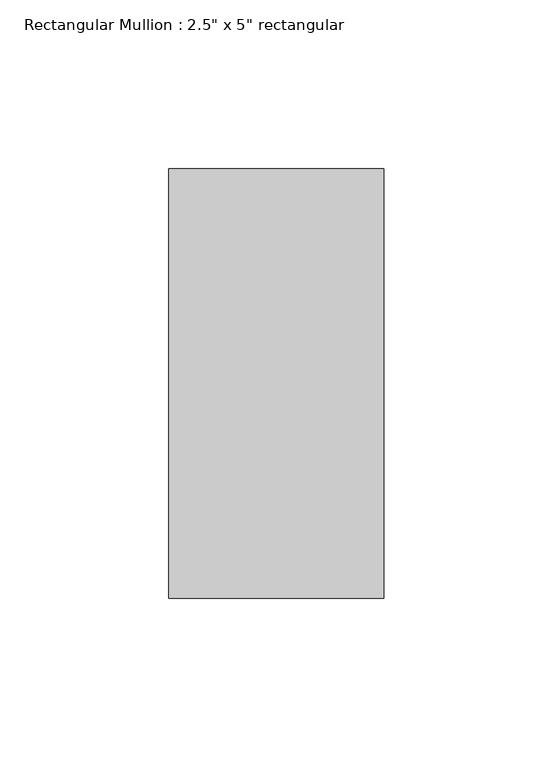
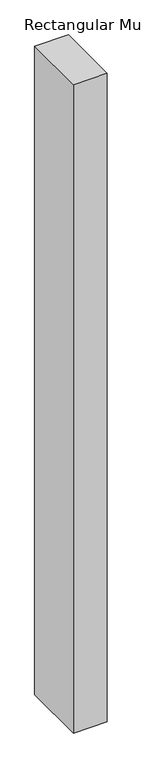
"""IFC4 building model written with IfcOpenShell, lengths in millimetres: member geometry."""

from ifc_helpers import new_model, si_unit, frame, origin, place, context, project, spatial, polyline, outline, extrude, source, transform, mapped, element, save


def member_c8c2a2fa(model_context):
    return source(origin(), model_context, "Body", "SweptSolid", [
        extrude(outline(polyline([(31.75, 63.5), (31.75, -63.5), (-31.75, -63.5), (-31.75, 63.5), (31.75, 63.5)])), frame((0.0, 0.0, -1295.4), z_axis=(0.0, 0.0, 1.0), x_axis=(1.0, 0.0, 0.0)), (0.0, 0.0, 1.0), 1295.4),
    ])


if __name__ == "__main__":
    model = new_model("IFC4")
    model_context = context("Model", 3, world=origin())
    ifc_project = project(units=[si_unit("LENGTHUNIT", "METRE", prefix="MILLI")], contexts=[model_context])
    site = spatial("IfcSite", under=ifc_project)
    building = spatial("IfcBuilding", under=site)
    placement = place(None, origin())
    member_shape = member_c8c2a2fa(model_context)
    element("IfcMember", 1, ObjectType="Rectangular Mullion : 2.5\" x 5\" rectangular", at=placement, inside=building, context=model_context, shape_type="MappedRepresentation", body=[
        mapped(member_shape, transform((0.0, 0.0, 0.0), x_axis=(1.0, 0.0, 0.0), y_axis=(0.0, 1.0, 0.0), z_axis=(0.0, 0.0, 1.0))),
    ])
    save(model, "model.ifc")

# Revit data of these elements
# Type "Rectangular Mullion : 2.5\" x 5\" rectangular"
#   built-in parameter 1007304 = 0.416667 (stored number, unit not read)
#   built-in parameter 1007301 = 0.104167 (stored number, unit not read)
#   built-in parameter 1007300 = 0.104167 (stored number, unit not read)
# Element 1 (IfcMember, "Rectangular Mullion : 2.5\" x 5\" rectangular")
#   Materials on its faces: "Aluminum"
# Materials
#   "Aluminum": class "Metal", colour RGB 247 247 247, transparency 0, Description = "Aluminum 6061", Cost = 0
